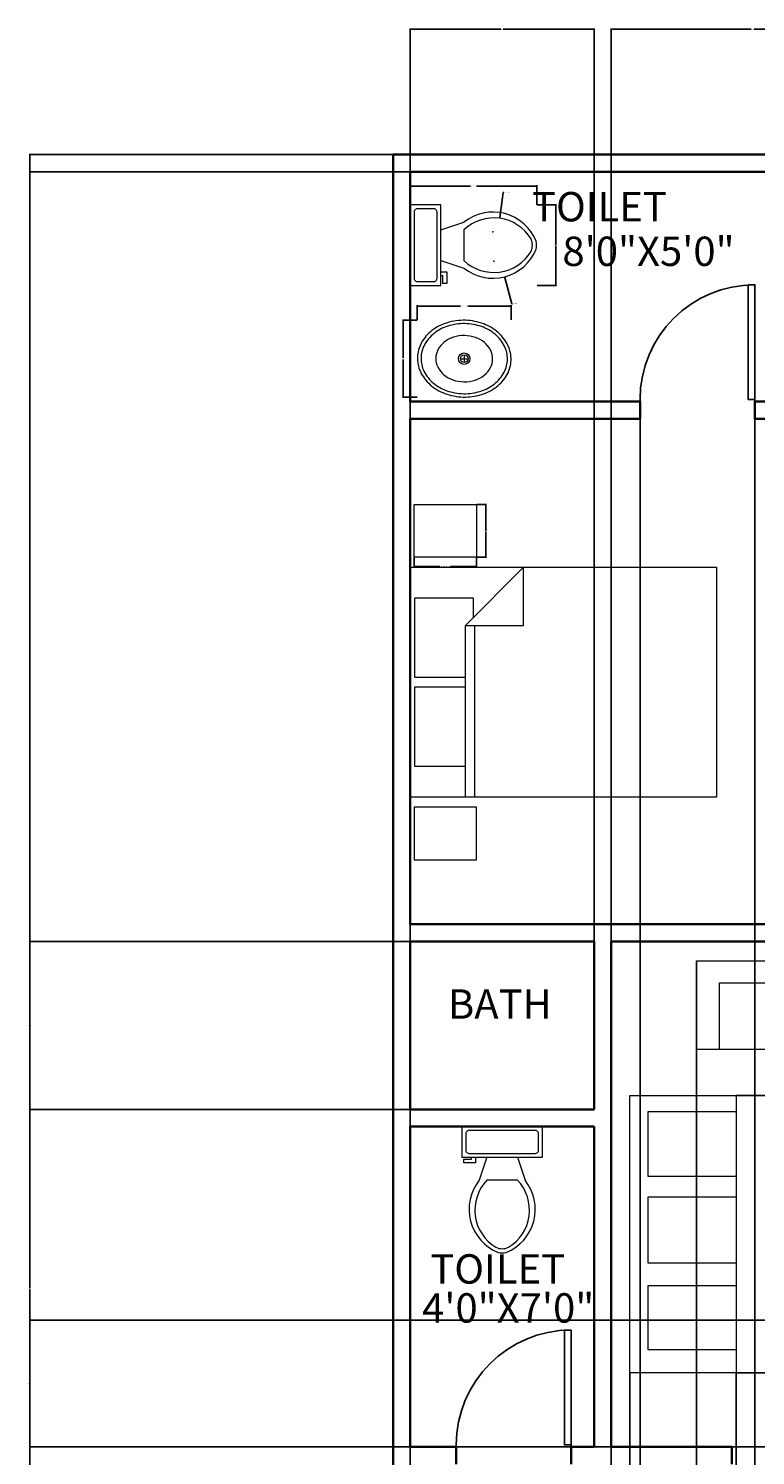
# Model space of a CAD drawing. Units: inches. Extents: x 2337 to 2851, y 1463 to 2183.
# Tile 2 of 4: x 2337 to 2527, y 1810 to 2183. Entities that reach past the tile are written whole.
import ezdxf

# ---------------------------------------------------------------- set-up
doc = ezdxf.new("R2010")
doc.units = ezdxf.units.IN
for name, color, linetype, lineweight in [('A-ANNO-DIMS', 2, 'Continuous', 18), ('A-AREA-IDEN', 7, 'Continuous', 18), ('A-DOOR', 4, 'Continuous', 25), ('A-FLOR-FIXT', 9, 'Continuous', 18), ('A-FURN', 8, 'Continuous', 18), ('A-WALL', 7, 'Continuous', 35)]:
    doc.layers.add(name, color=color, linetype=linetype, lineweight=lineweight)
doc.styles.get("Standard").update_dxf_attribs({"font": 'arial.ttf'})
doc.dimstyles.get("Standard").update_dxf_attribs({"dimtxt": 0.18, "dimasz": 0.18, "dimexe": 0.18, "dimexo": 0.0625, "dimgap": 0.09, "dimtad": 0, "dimtih": 1, "dimtoh": 1, "dimdec": 4, "dimzin": 0, "dimdsep": 46, "dimtxsty": 'Standard', "dimcen": 0.09, "dimadec": 0, "dimazin": 0, "dimtfac": 1, "dimtdec": 4, "dimtofl": 0, "dimtmove": 0, "dimatfit": 3, "dimfxl": 1, "dimtolj": 1, "dimtzin": 0, "dimarcsym": 0})

# ---------------------------------------------------------------- blocks, each defined once
blk = doc.blocks.new('*U2')
for p, q in [((0, 0), (0, -5)), ((30, 0), (30, -5))]:
    blk.add_line(p, q)
blk.add_lwpolyline([(0, 0), (0, 30), (1.75, 30), (1.75, 0)], close=True)
blk.add_arc((0, 0), 30, 0, 90)
blk = doc.blocks.new('Toilet - top')
for p, q in [((9.5, -6), (9.5, -2)), ((-10, -8.5), (-8, -8.5)), ((-10, -9.5), (-10, -8.5)), ((-7, -9.5), (-10, -9.5)), ((-8, -8.5), (-8, -8)), ((-7, -8), (-7, -9.5)), ((-4, -8), (-6, -14)), ((4, -8), (6, -14)), ((4, -14), (-4, -14))]:
    blk.add_line(p, q)
blk.add_lwpolyline([(10.5, -8), (10.5, 0), (-10.5, 0), (-10.5, -8)], close=True)
for points in [[(-9.5, -2), (-9.5, -6)], [(8.5, -1), (-8.5, -1)], [(-8.5, -7), (8.5, -7)]]:
    blk.add_lwpolyline(points)
for centre, radius, start, end in [((-8.62, -1.88), 0.884, 81.8699, 188.1301), ((8.62, -1.88), 0.884, 351.8699, 98.1301), ((-8.62, -6.12), 0.884, 171.8699, 278.1301), ((8.62, -6.12), 0.884, 261.8699, 8.1301), ((3.52, -21.58), 12.17, 141.4691, 247.9714), ((4.2, -21.82), 11.33, 136.3677, 238.9468), ((-3.52, -21.58), 12.17, 292.0284, 38.5307), ((-4.2, -21.82), 11.33, 301.053, 43.6321), ((0, -27.88), 4, 245.7318, 294.2682), ((0, -29), 4, 254.8605, 285.1395)]:
    blk.add_arc(centre, radius, start, end)
blk = doc.blocks.new('Sink - Oval top')
for p, q in [((-1, 0), (1, 0)), ((0, 1), (0, -1))]:
    blk.add_line(p, q)
for points in [[(-12.23, 0.39, 0.117634), (-11.46, -3.36, 0.104469), (-8.88, -6.8, 0.090016), (-5.08, -9.07, 0.08192), (-0.32, -10.02, 0.08192), (4.49, -9.38, 0.090016), (8.42, -7.36, 0.104469), (11.22, -4.09, 0.117634), (12.23, -0.39, 0.117634), (11.46, 3.36, 0.104469), (8.88, 6.8, 0.090016), (5.08, 9.07, 0.08192), (0.32, 10.02, 0.08192), (-4.49, 9.38, 0.090016), (-8.42, 7.36, 0.104469), (-11.22, 4.09, 0.117634)], [(-11.29, 0.16, 0.118622), (-10.52, -3.25, 0.104678), (-8.07, -6.36, 0.089562), (-4.54, -8.37, 0.081185), (-0.13, -9.15, 0.081185), (4.3, -8.49, 0.089562), (7.89, -6.58, 0.104678), (10.42, -3.55, 0.118622), (11.29, -0.16, 0.118622), (10.52, 3.25, 0.104678), (8.07, 6.36, 0.089562), (4.54, 8.37, 0.081185), (0.13, 9.15, 0.081185), (-4.3, 8.49, 0.089562), (-7.89, 6.58, 0.104678), (-10.42, 3.55, 0.118622)], [(-7.42, 0.08, 0.118283), (-6.91, -2.17, 0.104607), (-5.29, -4.21, 0.089718), (-2.97, -5.53, 0.081436), (-0.07, -6.04, 0.081436), (2.84, -5.59, 0.089718), (5.2, -4.33, 0.104607), (6.86, -2.32, 0.118283), (7.42, -0.08, 0.118283), (6.91, 2.17, 0.104607), (5.29, 4.21, 0.089718), (2.97, 5.53, 0.081436), (0.07, 6.04, 0.081436), (-2.84, 5.59, 0.089718), (-5.2, 4.33, 0.104607), (-6.86, 2.32, 0.118283)]]:
    blk.add_lwpolyline(points, format="xyb", close=True)
for radius in [1.5, 1]:
    blk.add_circle((0, 0), radius)
blk = doc.blocks.new('Bed - Queen')
for p, q in [((0, -80.00003), (0, 0)), ((0, 0), (59.99999, 0)), ((59.99999, 0), (59.99999, -80.00003)), ((7.99999, -1.2), (28.79998, -1.2)), ((7.99999, -14.4), (7.99999, -1.2)), ((28.79998, -1.2), (28.79998, -14.4)), ((31.19999, -1.2), (51.99999, -1.2)), ((31.19999, -14.4), (31.19999, -1.2)), ((51.99999, -1.2), (51.99999, -16.4)), ((0, -14.4), (44.8, -14.4)), ((59.99999, -29.6), (44.8, -14.4)), ((44.8, -14.4), (44.8, -29.6)), ((44.8, -16.8), (0, -16.8)), ((51.99999, -16.4), (46.79936, -16.4)), ((44.8, -29.6), (59.99999, -29.6)), ((59.99999, -80.00003), (0, -80.00003))]:
    blk.add_line(p, q)
blk = doc.blocks.new('NIGHTSTAND')
blk.add_lwpolyline([(0, 13.73), (16.32, 13.73), (16.32, 0), (0, 0)], close=True)
blk = doc.blocks.new('*D13')
at = {"layer": 'A-ANNO-DIMS', "color": 0, "lineweight": -2, "transparency": 16777216}
for p, q in [((2437.51, 2044.64), (2437.51, 2042.08)), ((2437.69, 2042.26), (2444.29, 2042.26)), ((2453.64, 2042.26), (2447.04, 2042.26)), ((2453.82, 2044.64), (2453.82, 2042.08))]:
    blk.add_line(p, q, dxfattribs=at)
at = {"layer": 'A-ANNO-DIMS', "color": 0, "transparency": 16777216}
for points in [[(2437.69, 2042.29), (2437.69, 2042.23), (2437.51, 2042.26)], [(2453.64, 2042.29), (2453.64, 2042.23), (2453.82, 2042.26)]]:
    blk.add_solid(points, dxfattribs=at)
at = {"layer": 'Defpoints', "color": 0, "transparency": 16777216}
for p in [(2437.51, 2044.7), (2453.82, 2044.7), (2453.82, 2042.26)]:
    blk.add_point(p, dxfattribs=at)
at = {"layer": 'A-ANNO-DIMS', "color": 0, "transparency": 16777216, "insert": (2445.66, 2042.26), "char_height": 0.18, "attachment_point": 5}
blk.add_mtext('\\A1;NIGHTSTAND 16 TYP.', dxfattribs=at)
blk = doc.blocks.new('*D14')
at = {"layer": 'A-ANNO-DIMS', "color": 0, "lineweight": -2, "transparency": 16777216}
for p, q in [((2453.89, 2058.43), (2456.45, 2058.43)), ((2456.27, 2058.25), (2456.27, 2051.75)), ((2456.27, 2044.88), (2456.27, 2051.39)), ((2453.89, 2044.7), (2456.45, 2044.7))]:
    blk.add_line(p, q, dxfattribs=at)
at = {"layer": 'A-ANNO-DIMS', "color": 0, "transparency": 16777216}
for points in [[(2456.24, 2058.25), (2456.3, 2058.25), (2456.27, 2058.43)], [(2456.24, 2044.88), (2456.3, 2044.88), (2456.27, 2044.7)]]:
    blk.add_solid(points, dxfattribs=at)
at = {"layer": 'Defpoints', "color": 0, "transparency": 16777216}
for p in [(2453.82, 2058.43), (2456.27, 2058.43), (2453.82, 2044.7)]:
    blk.add_point(p, dxfattribs=at)
at = {"layer": 'A-ANNO-DIMS', "color": 0, "transparency": 16777216, "insert": (2456.27, 2051.57), "char_height": 0.18, "attachment_point": 5}
blk.add_mtext('\\A1;14 TYP.', dxfattribs=at)
blk = doc.blocks.new('*D19')
at = {"layer": 'A-ANNO-DIMS', "color": 0, "lineweight": -2, "transparency": 16777216}
for p, q in [((2436.54, 2136.73), (2436.54, 2141.8)), ((2436.72, 2141.62), (2452.28, 2141.62)), ((2469.4, 2141.62), (2453.84, 2141.62)), ((2469.58, 2136.73), (2469.58, 2141.8))]:
    blk.add_line(p, q, dxfattribs=at)
at = {"layer": 'A-ANNO-DIMS', "color": 0, "transparency": 16777216}
for points in [[(2436.72, 2141.65), (2436.72, 2141.59), (2436.54, 2141.62)], [(2469.4, 2141.65), (2469.4, 2141.59), (2469.58, 2141.62)]]:
    blk.add_solid(points, dxfattribs=at)
at = {"layer": 'Defpoints', "color": 0, "transparency": 16777216}
for p in [(2436.54, 2141.62), (2436.54, 2136.67), (2469.58, 2136.67)]:
    blk.add_point(p, dxfattribs=at)
at = {"layer": 'A-ANNO-DIMS', "color": 0, "transparency": 16777216, "insert": (2453.06, 2141.62), "char_height": 0.18, "attachment_point": 5}
blk.add_mtext('\\A1;WC 33 TYP.', dxfattribs=at)
blk = doc.blocks.new('*D20')
at = {"layer": 'A-ANNO-DIMS', "color": 0, "lineweight": -2, "transparency": 16777216}
for p, q in [((2469.65, 2136.67), (2474.72, 2136.67)), ((2474.54, 2136.49), (2474.54, 2126.35)), ((2474.54, 2115.85), (2474.54, 2125.99)), ((2469.65, 2115.67), (2474.72, 2115.67))]:
    blk.add_line(p, q, dxfattribs=at)
at = {"layer": 'A-ANNO-DIMS', "color": 0, "transparency": 16777216}
for points in [[(2474.51, 2136.49), (2474.57, 2136.49), (2474.54, 2136.67)], [(2474.51, 2115.85), (2474.57, 2115.85), (2474.54, 2115.67)]]:
    blk.add_solid(points, dxfattribs=at)
at = {"layer": 'Defpoints', "color": 0, "transparency": 16777216}
for p in [(2469.58, 2136.67), (2474.54, 2136.67), (2469.58, 2115.67)]:
    blk.add_point(p, dxfattribs=at)
at = {"layer": 'A-ANNO-DIMS', "color": 0, "transparency": 16777216, "insert": (2474.54, 2126.17), "char_height": 0.18, "attachment_point": 5}
blk.add_mtext('\\A1;21 TYP.', dxfattribs=at)
blk = doc.blocks.new('*D21')
at = {"layer": 'A-ANNO-DIMS', "color": 0, "lineweight": -2, "transparency": 16777216}
for p, q in [((2438.35, 2106.66), (2438.35, 2110.46)), ((2438.53, 2110.28), (2449.69, 2110.28)), ((2462.72, 2110.28), (2451.56, 2110.28)), ((2462.9, 2106.66), (2462.9, 2110.46))]:
    blk.add_line(p, q, dxfattribs=at)
at = {"layer": 'A-ANNO-DIMS', "color": 0, "transparency": 16777216}
for points in [[(2438.53, 2110.31), (2438.53, 2110.25), (2438.35, 2110.28)], [(2462.72, 2110.31), (2462.72, 2110.25), (2462.9, 2110.28)]]:
    blk.add_solid(points, dxfattribs=at)
at = {"layer": 'Defpoints', "color": 0, "transparency": 16777216}
for p in [(2462.9, 2110.28), (2438.35, 2106.59), (2462.9, 2106.59)]:
    blk.add_point(p, dxfattribs=at)
at = {"layer": 'A-ANNO-DIMS', "color": 0, "transparency": 16777216, "insert": (2450.62, 2110.28), "char_height": 0.18, "attachment_point": 5}
blk.add_mtext('\\A1;BASIN 25 TYP.', dxfattribs=at)
blk = doc.blocks.new('*D22')
at = {"layer": 'A-ANNO-DIMS', "color": 0, "lineweight": -2, "transparency": 16777216}
for p, q in [((2438.29, 2106.59), (2434.49, 2106.59)), ((2434.67, 2106.41), (2434.67, 2096.71)), ((2434.67, 2086.64), (2434.67, 2096.34)), ((2438.29, 2086.46), (2434.49, 2086.46))]:
    blk.add_line(p, q, dxfattribs=at)
at = {"layer": 'A-ANNO-DIMS', "color": 0, "transparency": 16777216}
for points in [[(2434.64, 2106.41), (2434.7, 2106.41), (2434.67, 2106.59)], [(2434.64, 2086.64), (2434.7, 2086.64), (2434.67, 2086.46)]]:
    blk.add_solid(points, dxfattribs=at)
at = {"layer": 'Defpoints', "color": 0, "transparency": 16777216}
for p in [(2434.67, 2106.59), (2438.35, 2106.59), (2438.35, 2086.46)]:
    blk.add_point(p, dxfattribs=at)
at = {"layer": 'A-ANNO-DIMS', "color": 0, "transparency": 16777216, "insert": (2434.67, 2096.53), "char_height": 0.18, "attachment_point": 5}
blk.add_mtext('\\A1;20 TYP.', dxfattribs=at)
blk = doc.blocks.new('*D30')
at = {"layer": 'A-ANNO-DIMS', "color": 0, "lineweight": -2, "transparency": 16777216}
for p, q in [((2431.97, 2149.83), (2336.95, 2149.83)), ((2337.13, 2149.65), (2337.13, 1853.76)), ((2337.13, 1557.51), (2337.13, 1853.4)), ((2431.97, 1557.33), (2336.95, 1557.33))]:
    blk.add_line(p, q, dxfattribs=at)
at = {"layer": 'A-ANNO-DIMS', "color": 0, "transparency": 16777216}
for points in [[(2337.1, 2149.65), (2337.16, 2149.65), (2337.13, 2149.83)], [(2337.1, 1557.51), (2337.16, 1557.51), (2337.13, 1557.33)]]:
    blk.add_solid(points, dxfattribs=at)
at = {"layer": 'Defpoints', "color": 0, "transparency": 16777216}
for p in [(2337.13, 2149.83), (2432.04, 2149.83), (2432.04, 1557.33)]:
    blk.add_point(p, dxfattribs=at)
at = {"layer": 'A-ANNO-DIMS', "color": 0, "transparency": 16777216, "insert": (2337.13, 1853.58), "char_height": 0.18, "attachment_point": 5}
blk.add_mtext('\\A1;592.5', dxfattribs=at)
blk = doc.blocks.new('*D31')
at = {"layer": 'A-ANNO-DIMS', "color": 0, "lineweight": -2, "transparency": 16777216}
for p, q in [((2436.47, 1944.33), (2336.95, 1944.33)), ((2337.13, 1944.15), (2337.13, 1922.58)), ((2337.13, 1900.64), (2337.13, 1922.21)), ((2436.47, 1900.46), (2336.95, 1900.46))]:
    blk.add_line(p, q, dxfattribs=at)
at = {"layer": 'A-ANNO-DIMS', "color": 0, "transparency": 16777216}
for points in [[(2337.1, 1944.15), (2337.16, 1944.15), (2337.13, 1944.33)], [(2337.1, 1900.64), (2337.16, 1900.64), (2337.13, 1900.46)]]:
    blk.add_solid(points, dxfattribs=at)
at = {"layer": 'Defpoints', "color": 0, "transparency": 16777216}
for p in [(2436.54, 1944.33), (2337.13, 1900.46), (2436.54, 1900.46)]:
    blk.add_point(p, dxfattribs=at)
at = {"layer": 'A-ANNO-DIMS', "color": 0, "transparency": 16777216, "insert": (2337.13, 1922.4), "char_height": 0.18, "attachment_point": 5}
blk.add_mtext('\\A1;43.86', dxfattribs=at)
blk = doc.blocks.new('*D34')
at = {"layer": 'A-ANNO-DIMS', "color": 0, "lineweight": -2, "transparency": 16777216}
for p, q in [((2436.54, 1944.39), (2436.54, 2182.75)), ((2436.72, 2182.57), (2460.31, 2182.57)), ((2484.36, 2182.57), (2460.76, 2182.57)), ((2484.54, 1944.39), (2484.54, 2182.75))]:
    blk.add_line(p, q, dxfattribs=at)
at = {"layer": 'A-ANNO-DIMS', "color": 0, "transparency": 16777216}
for points in [[(2436.72, 2182.6), (2436.72, 2182.54), (2436.54, 2182.57)], [(2484.36, 2182.6), (2484.36, 2182.54), (2484.54, 2182.57)]]:
    blk.add_solid(points, dxfattribs=at)
at = {"layer": 'Defpoints', "color": 0, "transparency": 16777216}
for p in [(2484.54, 2182.57), (2436.54, 1944.33), (2484.54, 1944.33)]:
    blk.add_point(p, dxfattribs=at)
at = {"layer": 'A-ANNO-DIMS', "color": 0, "transparency": 16777216, "insert": (2460.54, 2182.57), "char_height": 0.18, "attachment_point": 5}
blk.add_mtext('\\A1;48', dxfattribs=at)
blk = doc.blocks.new('*D35')
at = {"layer": 'A-ANNO-DIMS', "color": 0, "lineweight": -2, "transparency": 16777216}
for p, q in [((2489.04, 1812.27), (2489.04, 1462.52)), ((2677.04, 1812.27), (2677.04, 1462.52)), ((2489.22, 1462.7), (2582.76, 1462.7)), ((2676.86, 1462.7), (2583.32, 1462.7))]:
    blk.add_line(p, q, dxfattribs=at)
at = {"layer": 'A-ANNO-DIMS', "color": 0, "transparency": 16777216}
for points in [[(2489.22, 1462.73), (2489.22, 1462.67), (2489.04, 1462.7)], [(2676.86, 1462.73), (2676.86, 1462.67), (2677.04, 1462.7)]]:
    blk.add_solid(points, dxfattribs=at)
at = {"layer": 'Defpoints', "color": 0, "transparency": 16777216}
for p in [(2489.04, 1812.33), (2677.04, 1812.33), (2677.04, 1462.7)]:
    blk.add_point(p, dxfattribs=at)
at = {"layer": 'A-ANNO-DIMS', "color": 0, "transparency": 16777216, "insert": (2583.04, 1462.7), "char_height": 0.18, "attachment_point": 5}
blk.add_mtext('\\A1;188', dxfattribs=at)
blk = doc.blocks.new('*D36')
at = {"layer": 'A-ANNO-DIMS', "color": 0, "lineweight": -2, "transparency": 16777216}
for p, q in [((2489.1, 1944.33), (2850.96, 1944.33)), ((2850.78, 1944.15), (2850.78, 1878.51)), ((2850.78, 1812.51), (2850.78, 1878.15)), ((2489.1, 1812.33), (2850.96, 1812.33))]:
    blk.add_line(p, q, dxfattribs=at)
at = {"layer": 'A-ANNO-DIMS', "color": 0, "transparency": 16777216}
for points in [[(2850.75, 1944.15), (2850.81, 1944.15), (2850.78, 1944.33)], [(2850.75, 1812.51), (2850.81, 1812.51), (2850.78, 1812.33)]]:
    blk.add_solid(points, dxfattribs=at)
at = {"layer": 'Defpoints', "color": 0, "transparency": 16777216}
for p in [(2489.04, 1944.33), (2850.78, 1944.33), (2489.04, 1812.33)]:
    blk.add_point(p, dxfattribs=at)
at = {"layer": 'A-ANNO-DIMS', "color": 0, "transparency": 16777216, "insert": (2850.78, 1878.33), "char_height": 0.18, "attachment_point": 5}
blk.add_mtext('\\A1;132', dxfattribs=at)
blk = doc.blocks.new('*D38')
at = {"layer": 'A-ANNO-DIMS', "color": 0, "lineweight": -2, "transparency": 16777216}
for p, q in [((2496.54, 2080.77), (2496.54, 1462.52)), ((2526.54, 2080.77), (2526.54, 1462.52)), ((2496.72, 1462.7), (2511.32, 1462.7)), ((2526.36, 1462.7), (2511.76, 1462.7))]:
    blk.add_line(p, q, dxfattribs=at)
at = {"layer": 'A-ANNO-DIMS', "color": 0, "transparency": 16777216}
for points in [[(2496.72, 1462.73), (2496.72, 1462.67), (2496.54, 1462.7)], [(2526.36, 1462.73), (2526.36, 1462.67), (2526.54, 1462.7)]]:
    blk.add_solid(points, dxfattribs=at)
at = {"layer": 'Defpoints', "color": 0, "transparency": 16777216}
for p in [(2496.54, 2080.83), (2526.54, 2080.83), (2526.54, 1462.7)]:
    blk.add_point(p, dxfattribs=at)
at = {"layer": 'A-ANNO-DIMS', "color": 0, "transparency": 16777216, "insert": (2511.54, 1462.7), "char_height": 0.18, "attachment_point": 5}
blk.add_mtext('\\A1;30', dxfattribs=at)
blk = doc.blocks.new('*D44')
at = {"layer": 'A-ANNO-DIMS', "color": 0, "lineweight": -2, "transparency": 16777216}
for p, q in [((2436.54, 2085.27), (2436.54, 1462.52)), ((2496.54, 2085.27), (2496.54, 1462.52)), ((2436.72, 1462.7), (2466.32, 1462.7)), ((2496.36, 1462.7), (2466.76, 1462.7))]:
    blk.add_line(p, q, dxfattribs=at)
at = {"layer": 'A-ANNO-DIMS', "color": 0, "transparency": 16777216}
for points in [[(2436.72, 1462.73), (2436.72, 1462.67), (2436.54, 1462.7)], [(2496.36, 1462.73), (2496.36, 1462.67), (2496.54, 1462.7)]]:
    blk.add_solid(points, dxfattribs=at)
at = {"layer": 'Defpoints', "color": 0, "transparency": 16777216}
for p in [(2436.54, 2085.33), (2496.54, 2085.33), (2496.54, 1462.7)]:
    blk.add_point(p, dxfattribs=at)
at = {"layer": 'A-ANNO-DIMS', "color": 0, "transparency": 16777216, "insert": (2466.54, 1462.7), "char_height": 0.18, "attachment_point": 5}
blk.add_mtext('\\A1;60', dxfattribs=at)
blk = doc.blocks.new('*D48')
at = {"layer": 'A-ANNO-DIMS', "color": 0, "lineweight": -2, "transparency": 16777216}
for p, q in [((2713.4, 1845.41), (2336.95, 1845.41)), ((2337.13, 1845.23), (2337.13, 1829.05)), ((2337.13, 1812.51), (2337.13, 1828.69)), ((2713.4, 1812.33), (2336.95, 1812.33))]:
    blk.add_line(p, q, dxfattribs=at)
at = {"layer": 'A-ANNO-DIMS', "color": 0, "transparency": 16777216}
for points in [[(2337.1, 1845.23), (2337.16, 1845.23), (2337.13, 1845.41)], [(2337.1, 1812.51), (2337.16, 1812.51), (2337.13, 1812.33)]]:
    blk.add_solid(points, dxfattribs=at)
at = {"layer": 'Defpoints', "color": 0, "transparency": 16777216}
for p in [(2337.13, 1845.41), (2713.47, 1845.41), (2713.47, 1812.33)]:
    blk.add_point(p, dxfattribs=at)
at = {"layer": 'A-ANNO-DIMS', "color": 0, "transparency": 16777216, "insert": (2337.13, 1828.87), "char_height": 0.18, "attachment_point": 5}
blk.add_mtext('\\A1;33.08', dxfattribs=at)
blk = doc.blocks.new('*D49')
at = {"layer": 'A-ANNO-DIMS', "color": 0, "lineweight": -2, "transparency": 16777216}
for p, q in [((2521.69, 1904.09), (2850.96, 1904.09)), ((2850.78, 1903.91), (2850.78, 1868.04)), ((2850.78, 1831.81), (2850.78, 1867.68)), ((2521.69, 1831.63), (2850.96, 1831.63))]:
    blk.add_line(p, q, dxfattribs=at)
at = {"layer": 'A-ANNO-DIMS', "color": 0, "transparency": 16777216}
for points in [[(2850.75, 1903.91), (2850.81, 1903.91), (2850.78, 1904.09)], [(2850.75, 1831.81), (2850.81, 1831.81), (2850.78, 1831.63)]]:
    blk.add_solid(points, dxfattribs=at)
at = {"layer": 'Defpoints', "color": 0, "transparency": 16777216}
for p in [(2521.63, 1904.09), (2850.78, 1904.09), (2521.63, 1831.63)]:
    blk.add_point(p, dxfattribs=at)
at = {"layer": 'A-ANNO-DIMS', "color": 0, "transparency": 16777216, "insert": (2850.78, 1867.86), "char_height": 0.18, "attachment_point": 5}
blk.add_mtext('\\A1;72.46', dxfattribs=at)
blk = doc.blocks.new('*D50')
at = {"layer": 'A-ANNO-DIMS', "color": 0, "lineweight": -2, "transparency": 16777216}
for p, q in [((2493.91, 1831.57), (2493.91, 1462.52)), ((2521.63, 1831.57), (2521.63, 1462.52)), ((2494.09, 1462.7), (2507.3, 1462.7)), ((2521.45, 1462.7), (2508.23, 1462.7))]:
    blk.add_line(p, q, dxfattribs=at)
at = {"layer": 'A-ANNO-DIMS', "color": 0, "transparency": 16777216}
for points in [[(2494.09, 1462.73), (2494.09, 1462.67), (2493.91, 1462.7)], [(2521.45, 1462.73), (2521.45, 1462.67), (2521.63, 1462.7)]]:
    blk.add_solid(points, dxfattribs=at)
at = {"layer": 'Defpoints', "color": 0, "transparency": 16777216}
for p in [(2493.91, 1831.63), (2521.63, 1831.63), (2521.63, 1462.7)]:
    blk.add_point(p, dxfattribs=at)
at = {"layer": 'A-ANNO-DIMS', "color": 0, "transparency": 16777216, "insert": (2507.77, 1462.7), "char_height": 0.18, "attachment_point": 5}
blk.add_mtext('\\A1;27.724', dxfattribs=at)
blk = doc.blocks.new('*D51')
at = {"layer": 'A-ANNO-DIMS', "color": 0, "lineweight": -2, "transparency": 16777216}
for p, q in [((2511.27, 1939.17), (2511.27, 1462.52)), ((2563.65, 1939.17), (2563.65, 1462.52)), ((2511.45, 1462.7), (2537.06, 1462.7)), ((2563.47, 1462.7), (2537.85, 1462.7))]:
    blk.add_line(p, q, dxfattribs=at)
at = {"layer": 'A-ANNO-DIMS', "color": 0, "transparency": 16777216}
for points in [[(2511.45, 1462.73), (2511.45, 1462.67), (2511.27, 1462.7)], [(2563.47, 1462.73), (2563.47, 1462.67), (2563.65, 1462.7)]]:
    blk.add_solid(points, dxfattribs=at)
at = {"layer": 'Defpoints', "color": 0, "transparency": 16777216}
for p in [(2511.27, 1939.23), (2563.65, 1939.23), (2563.65, 1462.7)]:
    blk.add_point(p, dxfattribs=at)
at = {"layer": 'A-ANNO-DIMS', "color": 0, "transparency": 16777216, "insert": (2537.46, 1462.7), "char_height": 0.18, "attachment_point": 5}
blk.add_mtext('\\A1;52.38', dxfattribs=at)
blk = doc.blocks.new('*D57')
at = {"layer": 'A-ANNO-DIMS', "color": 0, "lineweight": -2, "transparency": 16777216}
for p, q in [((2489.04, 1944.39), (2489.04, 2182.75)), ((2489.22, 2182.57), (2525.57, 2182.57)), ((2562.7, 2182.57), (2526.35, 2182.57)), ((2562.88, 1944.39), (2562.88, 2182.75))]:
    blk.add_line(p, q, dxfattribs=at)
at = {"layer": 'A-ANNO-DIMS', "color": 0, "transparency": 16777216}
for points in [[(2489.22, 2182.6), (2489.22, 2182.54), (2489.04, 2182.57)], [(2562.7, 2182.6), (2562.7, 2182.54), (2562.88, 2182.57)]]:
    blk.add_solid(points, dxfattribs=at)
at = {"layer": 'Defpoints', "color": 0, "transparency": 16777216}
for p in [(2562.88, 2182.57), (2489.04, 1944.33), (2562.88, 1944.33)]:
    blk.add_point(p, dxfattribs=at)
at = {"layer": 'A-ANNO-DIMS', "color": 0, "transparency": 16777216, "insert": (2525.96, 2182.57), "char_height": 0.18, "attachment_point": 5}
blk.add_mtext('\\A1;73.84', dxfattribs=at)
blk = doc.blocks.new('*D60')
at = {"layer": 'A-ANNO-DIMS', "color": 0, "lineweight": -2, "transparency": 16777216}
for p, q in [((2431.97, 2149.83), (2336.95, 2149.83)), ((2337.13, 2149.65), (2337.13, 2147.76)), ((2337.13, 2145.51), (2337.13, 2147.4)), ((2436.47, 2145.33), (2336.95, 2145.33))]:
    blk.add_line(p, q, dxfattribs=at)
at = {"layer": 'A-ANNO-DIMS', "color": 0, "transparency": 16777216}
for points in [[(2337.1, 2149.65), (2337.16, 2149.65), (2337.13, 2149.83)], [(2337.1, 2145.51), (2337.16, 2145.51), (2337.13, 2145.33)]]:
    blk.add_solid(points, dxfattribs=at)
at = {"layer": 'Defpoints', "color": 0, "transparency": 16777216}
for p in [(2432.04, 2149.83), (2337.13, 2145.33), (2436.54, 2145.33)]:
    blk.add_point(p, dxfattribs=at)
at = {"layer": 'A-ANNO-DIMS', "color": 0, "transparency": 16777216, "insert": (2337.13, 2147.58), "char_height": 0.18, "attachment_point": 5}
blk.add_mtext('\\A1;4.5', dxfattribs=at)
blk = doc.blocks.new('*D62')
at = {"layer": 'A-ANNO-DIMS', "color": 0, "lineweight": -2, "transparency": 16777216}
for p, q in [((2458.03, 2129.69), (2458.21, 2129.69)), ((2458.12, 2129.6), (2458.12, 2129.78)), ((2463.07, 2110.86), (2461.26, 2117.74)), ((2463.25, 2110.86), (2463.07, 2110.86))]:
    blk.add_line(p, q, dxfattribs=at)
at = {"layer": 'A-ANNO-DIMS', "color": 0, "transparency": 16777216}
blk.add_solid([(2461.28, 2117.75), (2461.23, 2117.74), (2461.21, 2117.92)], dxfattribs=at)
at = {"layer": 'Defpoints', "color": 0, "transparency": 16777216}
for p in [(2458.12, 2129.69), (2461.21, 2117.92)]:
    blk.add_point(p, dxfattribs=at)
at = {"layer": 'A-ANNO-DIMS', "color": 0, "transparency": 16777216, "insert": (2463.92, 2110.86), "char_height": 0.18, "attachment_point": 5}
blk.add_mtext('\\A1;4X R12.17', dxfattribs=at)
blk = doc.blocks.new('*D63')
at = {"layer": 'A-ANNO-DIMS', "color": 0, "lineweight": -2, "transparency": 16777216}
for p, q in [((2460.77, 2139.93), (2459.89, 2133.37)), ((2460.95, 2139.93), (2460.77, 2139.93)), ((2458.26, 2121.97), (2458.44, 2121.97)), ((2458.35, 2121.88), (2458.35, 2122.06))]:
    blk.add_line(p, q, dxfattribs=at)
at = {"layer": 'A-ANNO-DIMS', "color": 0, "transparency": 16777216}
blk.add_solid([(2459.86, 2133.38), (2459.92, 2133.37), (2459.86, 2133.2)], dxfattribs=at)
at = {"layer": 'Defpoints', "color": 0, "transparency": 16777216}
for p in [(2459.86, 2133.2), (2458.35, 2121.97)]:
    blk.add_point(p, dxfattribs=at)
at = {"layer": 'A-ANNO-DIMS', "color": 0, "transparency": 16777216, "insert": (2461.63, 2139.93), "char_height": 0.18, "attachment_point": 5}
blk.add_mtext('\\A1;4X R11.33', dxfattribs=at)

msp = doc.modelspace()

# ---------------------------------------------------------------- linework, layer by layer
at = {"layer": 'A-FURN'}
for points in [[(2511.2705, 1939.2296), (2563.646, 1939.2296), (2563.646, 1916.1026), (2511.2705, 1916.1026)], [(2517.311, 1933.4786), (2534.5678, 1933.4786), (2534.5678, 1916.1026), (2517.311, 1916.1026)], [(2493.9066, 1904.0882), (2521.6304, 1904.0882), (2521.6304, 1831.6316), (2493.9066, 1831.6316)], [(2498.6814, 1899.8866), (2521.6304, 1899.8866), (2521.6304, 1882.9741), (2498.6814, 1882.9741)], [(2498.6814, 1877.6548), (2521.6304, 1877.6548), (2521.6304, 1860.3241), (2498.6814, 1860.3241)], [(2498.6814, 1854.4541), (2521.6304, 1854.4541), (2521.6304, 1837.6825), (2498.6814, 1837.6825)]]:
    msp.add_lwpolyline(points, close=True, dxfattribs=at)
at = {"layer": 'A-WALL'}
for p, q in [((2432.0375, 2149.828), (2818.0375, 2149.828)), ((2432.0375, 2149.828), (2432.0375, 1557.328)), ((2432.0375, 2149.828), (2818.0375, 2149.828)), ((2436.5375, 2145.328), (2436.5375, 2085.328)), ((2436.5375, 2145.328), (2532.5375, 2145.328)), ((2436.5375, 2085.328), (2496.5375, 2085.328)), ((2496.5375, 2085.328), (2496.5375, 2080.828)), ((2526.5375, 2085.328), (2526.5375, 2080.828)), ((2526.5375, 2085.328), (2621.0375, 2085.328)), ((2436.5375, 2080.828), (2496.5375, 2080.828)), ((2436.5375, 2080.828), (2436.5375, 1948.828)), ((2526.5375, 2080.828), (2610.5375, 2080.828)), ((2436.5375, 1948.828), (2562.8796, 1948.828)), ((2436.5375, 1944.328), (2484.5375, 1944.328)), ((2436.5375, 1944.328), (2436.5375, 1900.4648)), ((2484.5375, 1944.328), (2484.5375, 1900.4648)), ((2489.0375, 1944.328), (2489.0375, 1812.328)), ((2489.0375, 1944.328), (2562.8796, 1944.328)), ((2436.5375, 1900.4648), (2484.5375, 1900.4648)), ((2436.5375, 1895.9648), (2484.5375, 1895.9648)), ((2436.5375, 1895.9648), (2436.5375, 1812.328)), ((2484.5375, 1895.9648), (2484.5375, 1812.328)), ((2436.5375, 1812.328), (2448.5375, 1812.328)), ((2448.5375, 1812.328), (2448.5375, 1807.828)), ((2478.5375, 1812.328), (2478.5375, 1807.828)), ((2478.5375, 1812.328), (2484.5375, 1812.328)), ((2489.0375, 1812.328), (2520.5375, 1812.328)), ((2520.5375, 1807.828), (2520.5375, 1812.328))]:
    msp.add_line(p, q, dxfattribs=at)

# ---------------------------------------------------------------- block references
at = {"layer": 'A-DOOR', "xscale": -1}
for p in [(2526.5375, 2085.828), (2478.5375, 1812.828)]:
    msp.add_blockref('*U2', p, dxfattribs=at)
at = {"layer": 'A-FLOR-FIXT', "rotation": 90}
msp.add_blockref('Toilet - top', (2436.5375, 2126.1668), dxfattribs=at)
at = {"layer": 'A-FLOR-FIXT'}
for name, p in [('Sink - Oval top', (2450.6234, 2096.5253)), ('Toilet - top', (2460.5375, 1895.9648))]:
    msp.add_blockref(name, p, dxfattribs=at)
at = {"layer": 'A-FURN'}
msp.add_blockref('NIGHTSTAND', (2437.506, 2044.705), dxfattribs=at)
at = {"layer": 'A-FURN', "rotation": 90}
msp.add_blockref('Bed - Queen', (2436.5375, 1982.0338), dxfattribs=at)
at = {"layer": 'A-FURN', "extrusion": (0, 0, -1), "zscale": -1, "rotation": 180}
msp.add_blockref('NIGHTSTAND', (-2437.506, 1979.3626), dxfattribs=at)

# ---------------------------------------------------------------- texts
at = {"layer": 'A-AREA-IDEN'}
for s, p in [('TOILET', (2468.3355, 2132.3847)), ('8\'0"X5\'0"', (2476.2637, 2120.733)), ('BATH', (2446.3666, 1924.1301)), ('TOILET', (2441.7652, 1854.9494)), ('4\'0"X7\'0"', (2439.6097, 1844.7715))]:
    msp.add_text(s, height=7.67227, dxfattribs=at).set_placement(p)

# ---------------------------------------------------------------- dimensions: what is measured, and where the dimension line sits
at = {"layer": 'A-ANNO-DIMS'}
for base, p1, p2, override, picture, middle in [((2484.5375, 2182.568), (2436.5375, 1944.328), (2484.5375, 1944.328), {"dimdec": 0, "dimlfac": 1, "dimrnd": 0, "dimzin": 0, "dimdsep": 46, "dimlunit": 2}, '*D34', (2460.5375, 2182.568)), ((2562.8796, 2182.568), (2489.0375, 1944.328), (2562.8796, 1944.328), {"dimdec": 2, "dimlfac": 1, "dimrnd": 0, "dimzin": 0, "dimdsep": 46, "dimlunit": 2}, '*D57', (2525.9585, 2182.568)), ((2496.5375, 1462.7036), (2436.5375, 2085.328), (2496.5375, 2085.328), {"dimdec": 0, "dimlfac": 1, "dimrnd": 0, "dimzin": 0, "dimdsep": 46, "dimlunit": 2}, '*D44', (2466.5375, 1462.7036)), ((2526.5375, 1462.7036), (2496.5375, 2080.828), (2526.5375, 2080.828), {"dimdec": 0, "dimlfac": 1, "dimrnd": 0, "dimzin": 0, "dimdsep": 46, "dimlunit": 2}, '*D38', (2511.5375, 1462.7036)), ((2563.646, 1462.7036), (2511.2705, 1939.2296), (2563.646, 1939.2296), {"dimdec": 2, "dimlfac": 1, "dimrnd": 0, "dimzin": 0, "dimdsep": 46, "dimlunit": 2}, '*D51', (2537.4582, 1462.7036)), ((2521.6304, 1462.7036), (2493.9066, 1831.6316), (2521.6304, 1831.6316), {"dimdec": 3, "dimlfac": 1, "dimrnd": 0, "dimzin": 0, "dimdsep": 46, "dimlunit": 2}, '*D50', (2507.7685, 1462.7036)), ((2677.0375, 1462.7036), (2489.0375, 1812.328), (2677.0375, 1812.328), {"dimdec": 0, "dimlfac": 1, "dimrnd": 0, "dimzin": 0, "dimdsep": 46, "dimlunit": 2}, '*D35', (2583.0375, 1462.7036))]:
    dim = msp.add_linear_dim(base=base, p1=p1, p2=p2, dimstyle='Standard', override=override, dxfattribs=at)
    dim.commit()
    dim.dimension.update_dxf_attribs({"geometry": picture, "text_midpoint": middle})
for base, p1, p2, override, picture, middle in [((2337.1275, 2149.828), (2432.0375, 1557.328), (2432.0375, 2149.828), {"dimdec": 1, "dimlfac": 1, "dimrnd": 0, "dimzin": 0, "dimdsep": 46, "dimlunit": 2}, '*D30', (2337.1275, 1853.578)), ((2337.1275, 2145.328), (2432.0375, 2149.828), (2436.5375, 2145.328), {"dimdec": 1, "dimlfac": 1, "dimrnd": 0, "dimzin": 0, "dimdsep": 46, "dimlunit": 2}, '*D60', (2337.1275, 2147.578)), ((2337.1275, 1900.4648), (2436.5375, 1944.328), (2436.5375, 1900.4648), {"dimdec": 2, "dimlfac": 1, "dimrnd": 0, "dimzin": 0, "dimdsep": 46, "dimlunit": 2}, '*D31', (2337.1275, 1922.3964)), ((2850.7775, 1944.328), (2489.0375, 1812.328), (2489.0375, 1944.328), {"dimdec": 0, "dimlfac": 1, "dimrnd": 0, "dimzin": 0, "dimdsep": 46, "dimlunit": 2}, '*D36', (2850.7775, 1878.328)), ((2850.7775, 1904.0882), (2521.6304, 1831.6316), (2521.6304, 1904.0882), {"dimdec": 2, "dimlfac": 1, "dimrnd": 0, "dimzin": 0, "dimdsep": 46, "dimlunit": 2}, '*D49', (2850.7775, 1867.8599)), ((2337.1275, 1845.4107), (2713.4656, 1812.328), (2713.4656, 1845.4107), {"dimdec": 2, "dimlfac": 1, "dimrnd": 0, "dimzin": 0, "dimdsep": 46, "dimlunit": 2}, '*D48', (2337.1275, 1828.8693))]:
    dim = msp.add_linear_dim(base=base, p1=p1, p2=p2, angle=90, dimstyle='Standard', override=override, dxfattribs=at)
    dim.commit()
    dim.dimension.update_dxf_attribs({"geometry": picture, "text_midpoint": middle})
for base, p1, p2, angle, text, picture, middle in [((2436.5375, 2141.6238), (2469.5837, 2136.6668), (2436.5375, 2136.6668), 180, 'WC <> TYP.', '*D19', (2453.0606, 2141.6238)), ((2474.5406, 2136.6668), (2469.5837, 2115.6668), (2469.5837, 2136.6668), 90, '<> TYP.', '*D20', (2474.5406, 2126.1668)), ((2434.6654, 2106.5936), (2438.348, 2086.457), (2438.348, 2106.5936), 90, '<> TYP.', '*D22', (2434.6654, 2096.5253)), ((2456.2703, 2058.4312), (2453.8229, 2044.705), (2453.8229, 2058.4312), 90, '<> TYP.', '*D14', (2456.2703, 2051.5681))]:
    dim = msp.add_linear_dim(base=base, p1=p1, p2=p2, angle=angle, text=text, dimstyle='Standard', override={"dimdec": 0, "dimlfac": 1, "dimrnd": 0, "dimzin": 0, "dimdsep": 46, "dimlunit": 2}, dxfattribs=at)
    dim.commit()
    dim.dimension.update_dxf_attribs({"geometry": picture, "text_midpoint": middle})
for center, mpoint, picture, middle in [((2458.3548, 2121.9669), (2459.864, 2133.1952), '*D63', (2461.6264, 2139.9321)), ((2458.1179, 2129.6864), (2461.2101, 2117.9168), '*D62', (2463.9222, 2110.855))]:
    dim = msp.add_radius_dim(center=center, mpoint=mpoint, text='4X <>', dimstyle='Standard', override={"dimdec": 2, "dimlfac": 1, "dimrnd": 0, "dimzin": 0, "dimdsep": 46, "dimlunit": 2}, dxfattribs=at)
    dim.commit()
    dim.dimension.update_dxf_attribs({"geometry": picture, "text_midpoint": middle, "dimtype": 164})
for base, p1, p2, text, picture, middle in [((2462.8989, 2110.2762), (2438.348, 2106.5936), (2462.8989, 2106.5936), 'BASIN <> TYP.', '*D21', (2450.6234, 2110.2762)), ((2453.8229, 2042.2575), (2437.5064, 2044.705), (2453.8229, 2044.705), 'NIGHTSTAND <> TYP.', '*D13', (2445.6646, 2042.2575))]:
    dim = msp.add_linear_dim(base=base, p1=p1, p2=p2, text=text, dimstyle='Standard', override={"dimdec": 0, "dimlfac": 1, "dimrnd": 0, "dimzin": 0, "dimdsep": 46, "dimlunit": 2}, dxfattribs=at)
    dim.commit()
    dim.dimension.update_dxf_attribs({"geometry": picture, "text_midpoint": middle})

doc.saveas('drawing.dxf')
